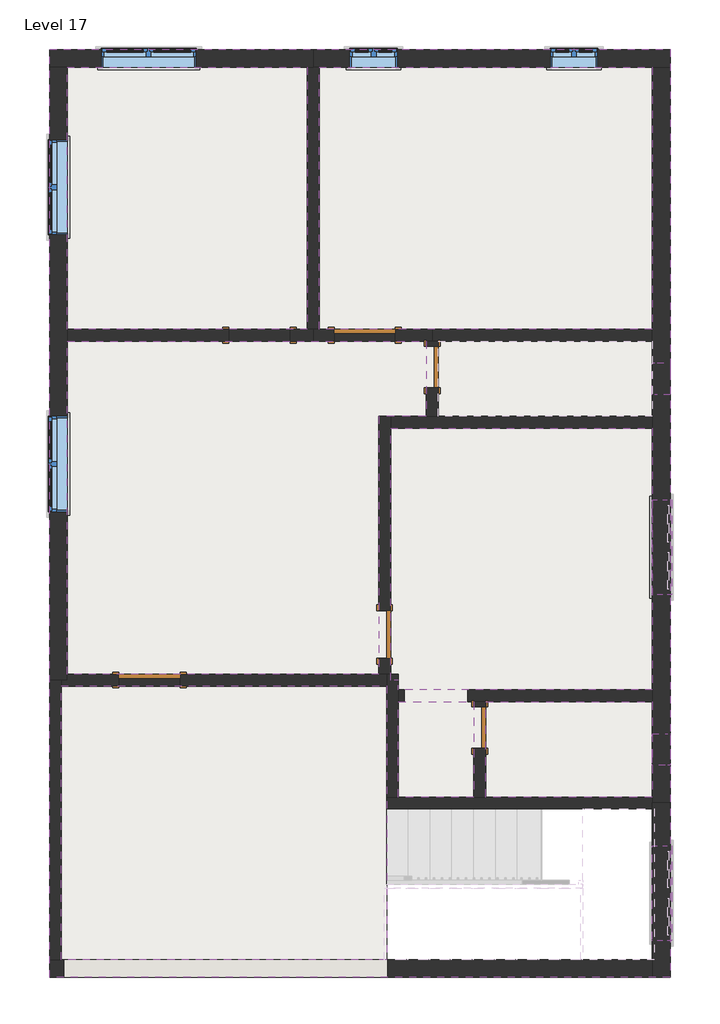
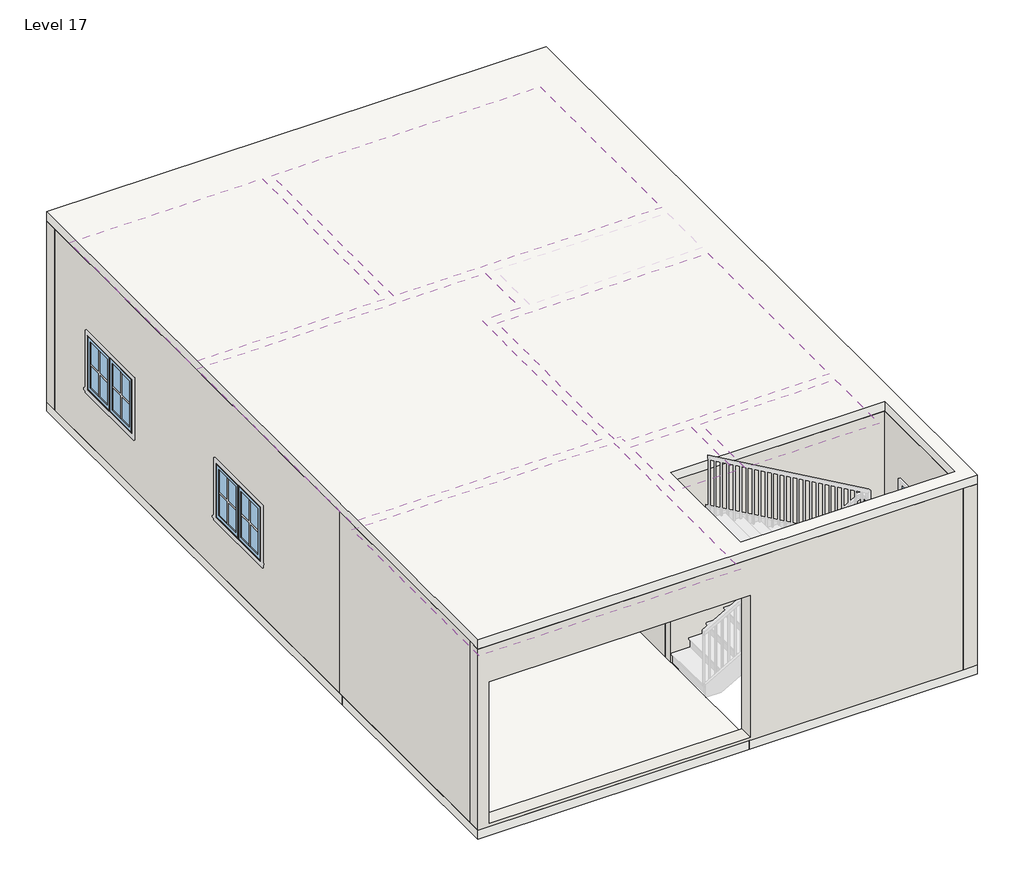
# One storey, part 1 of 2: 27 walls, 13 windows, 7 coverings, 6 doors, 3 slabs.
"""IFC4 building model written with IfcOpenShell, lengths in millimetres."""

from ifc_helpers import new_model, si_unit, frame, origin, place, context, project, spatial, polyline, outline, extrude, faceted_brep, transform, mapped, element, save
from components import door_2908be75, door_9ea4ff49, door_dc34e247, door_b804d09e, fixed_2_415b3208, window_casement_double_3_c417fced, window_casement_double_4_c19c33cb

model = new_model("IFC4")

# Units and contexts
model_context = context("Model", 3, world=origin())
ifc_project = project(units=[si_unit("LENGTHUNIT", "METRE", prefix="MILLI")], contexts=[model_context])

# Site, building, storey
site = spatial("IfcSite", under=ifc_project)
building = spatial("IfcBuilding", under=site)
storey = spatial("IfcBuildingStorey", under=building, Name="Level 17", Elevation=9601.2)

# Coverings
placement = place(None, origin())
element("IfcCovering", 1, ObjectType="2' x 4' ACT System", at=placement, inside=storey, context=model_context, shape_type="SweptSolid", body=[
    extrude(outline(polyline([(-5680.5154463, 2323.8455275), (-5680.5154463, 5678.2330275), (-2607.1154463, 5678.2330275), (-2607.1154463, 2323.8455275), (-5680.5154463, 2323.8455275)])), frame((0.0, 0.0, 12344.4), z_axis=(0.0, 0.0, 1.0), x_axis=(1.0, 0.0, 0.0)), (0.0, 0.0, 1.0), 57.15),
])
element("IfcCovering", 2, ObjectType="2' x 4' ACT System", at=placement, inside=storey, context=model_context, shape_type="SweptSolid", body=[
    extrude(outline(polyline([(-2454.7154463, 2323.8455275), (-2454.7154463, 5678.2330275), (1812.4845537, 5678.2330275), (1812.4845537, 2323.8455275), (-2454.7154463, 2323.8455275)])), frame((0.0, 0.0, 12344.4), z_axis=(0.0, 0.0, 1.0), x_axis=(1.0, 0.0, 0.0)), (0.0, 0.0, 1.0), 57.15),
])
element("IfcCovering", 3, ObjectType="2' x 4' ACT System", at=placement, inside=storey, context=model_context, shape_type="SweptSolid", body=[
    extrude(outline(polyline([(-5680.5154463, -2095.7544725), (-5680.5154463, 2171.4455275), (-1083.1154463, 2171.4455275), (-1083.1154463, 1206.2455275), (-1692.7154463, 1206.2455275), (-1692.7154463, -2095.7544725), (-5680.5154463, -2095.7544725)])), frame((0.0, 0.0, 12344.4), z_axis=(0.0, 0.0, 1.0), x_axis=(1.0, 0.0, 0.0)), (0.0, 0.0, 1.0), 57.15),
])
element("IfcCovering", 4, ObjectType="2' x 4' ACT System", at=placement, inside=storey, context=model_context, shape_type="SweptSolid", body=[
    extrude(outline(polyline([(1812.4845537, 1053.8455275), (1812.4845537, -2298.9544725), (-1438.7154463, -2298.9544725), (-1438.7154463, -2171.9544725), (-1540.3154463, -2171.9544725), (-1540.3154463, 1053.8455275), (1812.4845537, 1053.8455275)])), frame((0.0, 0.0, 12344.4), z_axis=(0.0, 0.0, 1.0), x_axis=(1.0, 0.0, 0.0)), (0.0, 0.0, 1.0), 57.15),
])
element("IfcCovering", 5, ObjectType="2' x 4' ACT System", at=placement, inside=storey, context=model_context, shape_type="SweptSolid", body=[
    extrude(outline(polyline([(1812.4845537, -2451.3544725), (1812.4845537, -3670.5544725), (-321.1154463, -3670.5544725), (-321.1154463, -2451.3544725), (1812.4845537, -2451.3544725)])), frame((0.0, 0.0, 12344.4), z_axis=(0.0, 0.0, 1.0), x_axis=(1.0, 0.0, 0.0)), (0.0, 0.0, 1.0), 57.15),
])
element("IfcCovering", 6, ObjectType="2' x 4' ACT System", at=placement, inside=storey, context=model_context, shape_type="SweptSolid", body=[
    extrude(outline(polyline([(-473.5154463, -2451.3544725), (-473.5154463, -3670.5544725), (-1438.7154463, -3670.5544725), (-1438.7154463, -2451.3544725), (-473.5154463, -2451.3544725)])), frame((0.0, 0.0, 12344.4), z_axis=(0.0, 0.0, 1.0), x_axis=(1.0, 0.0, 0.0)), (0.0, 0.0, 1.0), 57.15),
])
element("IfcCovering", 7, ObjectType="2' x 4' ACT System", at=placement, inside=storey, context=model_context, shape_type="SweptSolid", body=[
    extrude(outline(polyline([(-1591.1154463, -2248.1544725), (-1591.1154463, -5753.3544725), (-5756.7154463, -5753.3544725), (-5756.7154463, -2248.1544725), (-1591.1154463, -2248.1544725)])), frame((0.0, 0.0, 12344.4), z_axis=(0.0, 0.0, 1.0), x_axis=(1.0, 0.0, 0.0)), (0.0, 0.0, 1.0), 57.15),
])

# Doors
door_shape = door_2908be75(model_context)
element("IfcDoor", 8, ObjectType="Single-Flush : 1' 9\"", at=placement, inside=storey, context=model_context, shape_type="MappedRepresentation", body=[
    mapped(door_shape, transform((-397.3154463, -2781.5544725, 9601.2), x_axis=(0.0, 1.0, 0.0), y_axis=(-1.0, 0.0, 0.0), z_axis=(0.0, 0.0, 1.0))),
])
element("IfcDoor", 9, ObjectType="Single-Flush : 1' 9\"", at=placement, inside=storey, context=model_context, shape_type="MappedRepresentation", body=[
    mapped(door_shape, transform((-1006.9154463, 1841.2455275, 9601.2), x_axis=(0.0, 1.0, 0.0), y_axis=(-1.0, 0.0, 0.0), z_axis=(0.0, 0.0, 1.0))),
])
door_2_shape = door_9ea4ff49(model_context)
element("IfcDoor", 10, ObjectType="Single-Flush : 2'0\"", at=placement, inside=storey, context=model_context, shape_type="MappedRepresentation", body=[
    mapped(door_2_shape, transform((-1616.5154463, -1587.7544725, 9601.2), x_axis=(0.0, -1.0, 0.0), y_axis=(1.0, 0.0, 0.0), z_axis=(0.0, 0.0, 1.0))),
])
door_3_shape = door_dc34e247(model_context)
element("IfcDoor", 11, ObjectType="Single-Flush : 2'7\"", at=placement, inside=storey, context=model_context, shape_type="MappedRepresentation", body=[
    mapped(door_3_shape, transform((-4626.4154463, -2171.9544725, 9601.2), x_axis=(-1.0, 0.0, 0.0), y_axis=(0.0, -1.0, 0.0), z_axis=(0.0, 0.0, 1.0))),
])
element("IfcDoor", 12, ObjectType="Single-Flush : 2'7\"", at=placement, inside=storey, context=model_context, shape_type="MappedRepresentation", body=[
    mapped(door_3_shape, transform((-1870.5154463, 2247.6455275, 9601.2), x_axis=(-1.0, 0.0, 0.0), y_axis=(0.0, -1.0, 0.0), z_axis=(0.0, 0.0, 1.0))),
])
door_4_shape = door_b804d09e(model_context)
element("IfcDoor", 13, ObjectType="Single-Flush : 2'7\"", at=placement, inside=storey, context=model_context, shape_type="MappedRepresentation", body=[
    mapped(door_4_shape, transform((-3216.7154463, 2247.6455275, 9601.2), x_axis=(1.0, 0.0, 0.0), y_axis=(0.0, 1.0, 0.0), z_axis=(0.0, 0.0, 1.0))),
])

# Slabs
element("IfcSlab", 14, ObjectType="Generic - 6\"", at=placement, inside=storey, context=model_context, shape_type="SweptSolid", body=[
    extrude(outline(polyline([(-5909.1154463, -2248.1544725), (-5909.1154463, 5906.8330275), (2041.0845537, 5906.8330275), (2041.0845537, -5981.9544725), (-1591.1154463, -5981.9544725), (-1591.1154463, -5753.3544725), (1812.4845537, -5753.3544725), (1812.4845537, -3822.9544725), (-1591.1154463, -3822.9544725), (-1591.1154463, -2248.1544725), (-5756.7154463, -2248.1544725), (-5909.1154463, -2248.1544725)])), frame((0.0, 0.0, 9448.8), z_axis=(0.0, 0.0, 1.0), x_axis=(1.0, 0.0, 0.0)), (0.0, 0.0, 1.0), 152.4),
])
element("IfcSlab", 15, ObjectType="Generic - 6\"", at=placement, inside=storey, context=model_context, shape_type="SweptSolid", body=[
    extrude(outline(polyline([(-1591.1154463, -2248.1544725), (-1591.1154463, -5981.9544725), (-5909.1154463, -5981.9544725), (-5909.1154463, -2248.1544725), (-1591.1154463, -2248.1544725)])), frame((0.0, 0.0, 9448.8), z_axis=(0.0, 0.0, 1.0), x_axis=(1.0, 0.0, 0.0)), (0.0, 0.0, 1.0), 152.4),
])
element("IfcSlab", 16, ObjectType="Generic - 6\"", at=placement, inside=storey, context=model_context, shape_type="SweptSolid", body=[
    extrude(outline(polyline([(2041.0845537, 5906.8330275), (2041.0845537, -5981.9544725), (-5909.1154463, -5981.9544725), (-5909.1154463, 5906.8330275), (2041.0845537, 5906.8330275)]), holes=[polyline([(1812.4845537, -3822.9544725), (-1591.1154463, -3822.9544725), (-1591.1154463, -5753.3544725), (1812.4845537, -5753.3544725), (1812.4845537, -3822.9544725)])]), frame((0.0, 0.0, 12649.2), z_axis=(0.0, 0.0, 1.0), x_axis=(1.0, 0.0, 0.0)), (0.0, 0.0, 1.0), 152.4),
])

# Walls
element("IfcWall", 17, ObjectType="Generic - 6\"", at=placement, inside=storey, context=model_context, shape_type="Brep", body=[
    faceted_brep([(-5909.1154463, -2171.9544725, 9601.2), (-5909.1154463, -5753.3544725, 9601.2), (-5909.1154463, -5753.3544725, 12649.2), (-5909.1154463, -2171.9544725, 12649.2), (-5756.7154463, -2171.9544725, 9601.2), (-5756.7154463, -2171.9544725, 12649.2), (-5756.7154463, -2248.1544725, 12649.2), (-5756.7154463, -5753.3544725, 12649.2), (-5756.7154463, -5753.3544725, 9601.2), (-5756.7154463, -2248.1544725, 9601.2)], [[[0, 1, 2, 3]], [[4, 5, 6, 7, 8, 9]], [[1, 0, 4, 9, 8]], [[3, 2, 7, 6, 5]], [[0, 3, 5, 4]], [[2, 1, 8, 7]]]),
])
element("IfcWall", 18, ObjectType="Generic - 6\"", at=placement, inside=storey, context=model_context, shape_type="Brep", body=[
    faceted_brep([(1812.4845537, -3670.5544725, 9601.2), (-321.1154463, -3670.5544725, 9601.2), (-473.5154463, -3670.5544725, 9601.2), (-1438.7154463, -3670.5544725, 9601.2), (-1591.1154463, -3670.5544725, 9601.2), (-1591.1154463, -3670.5544725, 12649.2), (-1438.7154463, -3670.5544725, 12649.2), (-473.5154463, -3670.5544725, 12649.2), (-321.1154463, -3670.5544725, 12649.2), (1812.4845537, -3670.5544725, 12649.2), (1812.4845537, -3822.9544725, 9601.2), (1812.4845537, -3822.9544725, 12649.2), (-1591.1154463, -3822.9544725, 12649.2), (-1591.1154463, -3822.9544725, 9601.2), (1812.4845537, -3746.7544725, 9601.2), (1812.4845537, -3746.7544725, 12649.2)], [[[0, 1, 2, 3, 4, 5, 6, 7, 8, 9]], [[10, 11, 12, 13]], [[4, 3, 2, 1, 0, 14, 10, 13]], [[9, 8, 7, 6, 5, 12, 11, 15]], [[5, 4, 13, 12]], [[0, 9, 15, 11, 10, 14]]]),
])
element("IfcWall", 19, ObjectType="Generic - 6\"", at=placement, inside=storey, context=model_context, shape_type="Brep", body=[
    faceted_brep([(-1438.7154463, -3670.5544725, 9601.2), (-1438.7154463, -2451.3544725, 9601.2), (-1438.7154463, -2298.9544725, 9601.2), (-1438.7154463, -2095.7544725, 9601.2), (-1438.7154463, -2095.7544725, 12649.2), (-1438.7154463, -2298.9544725, 12649.2), (-1438.7154463, -2451.3544725, 12649.2), (-1438.7154463, -3670.5544725, 12649.2), (-1591.1154463, -3670.5544725, 9601.2), (-1591.1154463, -3670.5544725, 12649.2), (-1591.1154463, -2248.1544725, 12649.2), (-1591.1154463, -2171.9544725, 12649.2), (-1591.1154463, -2095.7544725, 12649.2), (-1591.1154463, -2095.7544725, 9601.2), (-1591.1154463, -2171.9544725, 9601.2), (-1591.1154463, -2248.1544725, 9601.2), (-1540.3154463, -2095.7544725, 9601.2), (-1540.3154463, -2095.7544725, 12649.2)], [[[0, 1, 2, 3, 4, 5, 6, 7]], [[8, 9, 10, 11, 12, 13, 14, 15]], [[3, 2, 1, 0, 8, 15, 14, 13, 16]], [[7, 6, 5, 4, 17, 12, 11, 10, 9]], [[0, 7, 9, 8]], [[4, 3, 16, 13, 12, 17]]]),
])
element("IfcWall", 20, ObjectType="Generic - 6\"", at=placement, inside=storey, context=model_context, shape_type="Brep", body=[
    faceted_brep([(-5020.1154463, -2095.7544725, 11734.8), (-5020.1154463, -2095.7544725, 9601.2), (-5680.5154463, -2095.7544725, 9601.2), (-5680.5154463, -2095.7544725, 12649.2), (-1692.7154463, -2095.7544725, 12649.2), (-1591.1154463, -2095.7544725, 12649.2), (-1591.1154463, -2095.7544725, 9601.2), (-1692.7154463, -2095.7544725, 9601.2), (-4232.7154463, -2095.7544725, 9601.2), (-4232.7154463, -2095.7544725, 11734.8), (-5756.7154463, -2248.1544725, 9601.2), (-5020.1154463, -2248.1544725, 9601.2), (-5020.1154463, -2248.1544725, 11734.8), (-4232.7154463, -2248.1544725, 11734.8), (-4232.7154463, -2248.1544725, 9601.2), (-1591.1154463, -2248.1544725, 9601.2), (-1591.1154463, -2248.1544725, 12649.2), (-5756.7154463, -2248.1544725, 12649.2), (-5756.7154463, -2171.9544725, 9601.2), (-5680.5154463, -2171.9544725, 9601.2), (-5680.5154463, -2171.9544725, 12649.2), (-5756.7154463, -2171.9544725, 12649.2)], [[[0, 1, 2, 3, 4, 5, 6, 7, 8, 9]], [[10, 11, 12, 13, 14, 15, 16, 17]], [[2, 1, 11, 10, 18, 19]], [[8, 7, 6, 15, 14]], [[5, 4, 3, 20, 21, 17, 16]], [[3, 2, 19, 20]], [[19, 18, 21, 20]], [[18, 10, 17, 21]], [[6, 5, 16, 15]], [[12, 11, 1, 0]], [[13, 12, 0, 9]], [[14, 13, 9, 8]]]),
])
element("IfcWall", 21, ObjectType="Generic - 6\"", at=placement, inside=storey, context=model_context, shape_type="Brep", body=[
    faceted_brep([(1812.4845537, -2451.3544725, 9601.2), (1812.4845537, -2451.3544725, 12649.2), (-321.1154463, -2451.3544725, 12649.2), (-473.5154463, -2451.3544725, 12649.2), (-1438.7154463, -2451.3544725, 12649.2), (-1438.7154463, -2451.3544725, 9601.2), (-1367.0206652, -2451.3544725, 9601.2), (-1367.0206652, -2451.3544725, 12039.6), (-547.4818767, -2451.3544725, 12039.6), (-547.4818767, -2451.3544725, 9601.2), (-473.5154463, -2451.3544725, 9601.2), (-321.1154463, -2451.3544725, 9601.2), (1812.4845537, -2298.9544725, 12649.2), (1812.4845537, -2298.9544725, 9601.2), (-547.4818767, -2298.9544725, 9601.2), (-547.4818767, -2298.9544725, 12039.6), (-1367.0206652, -2298.9544725, 12039.6), (-1367.0206652, -2298.9544725, 9601.2), (-1438.7154463, -2298.9544725, 9601.2), (-1438.7154463, -2298.9544725, 12649.2)], [[[0, 1, 2, 3, 4, 5, 6, 7, 8, 9, 10, 11]], [[12, 13, 14, 15, 16, 17, 18, 19]], [[5, 18, 17, 6]], [[13, 0, 11, 10, 9, 14]], [[4, 3, 2, 1, 12, 19]], [[1, 0, 13, 12]], [[5, 4, 19, 18]], [[7, 16, 15, 8]], [[16, 7, 6, 17]], [[8, 15, 14, 9]]]),
])
element("IfcWall", 22, ObjectType="Generic - 6\"", at=placement, inside=storey, context=model_context, shape_type="SweptSolid", body=[
    extrude(outline(polyline([(-2451.3544725, 9601.2), (-2514.8544725, 9601.2), (-2514.8544725, 11734.8), (-3048.2544725, 11734.8), (-3048.2544725, 9601.2), (-3670.5544725, 9601.2), (-3670.5544725, 12649.2), (-2451.3544725, 12649.2), (-2451.3544725, 9601.2)])), frame((-473.5154463, 0.0, 0.0), z_axis=(1.0, 0.0, 0.0), x_axis=(0.0, 1.0, 0.0)), (0.0, 0.0, 1.0), 152.4),
])
element("IfcWall", 23, ObjectType="Generic - 6\"", at=placement, inside=storey, context=model_context, shape_type="Brep", body=[
    faceted_brep([(-1540.3154463, -2095.7544725, 9601.2), (-1540.3154463, -1892.5544725, 9601.2), (-1540.3154463, -1892.5544725, 11734.8), (-1540.3154463, -1282.9544725, 11734.8), (-1540.3154463, -1282.9544725, 9601.2), (-1540.3154463, 1053.8455275, 9601.2), (-1540.3154463, 1206.2455275, 9601.2), (-1540.3154463, 1206.2455275, 12649.2), (-1540.3154463, 1053.8455275, 12649.2), (-1540.3154463, -2095.7544725, 12649.2), (-1692.7154463, -1892.5544725, 11734.8), (-1692.7154463, -1892.5544725, 9601.2), (-1692.7154463, -2095.7544725, 9601.2), (-1692.7154463, -2095.7544725, 12649.2), (-1692.7154463, 1206.2455275, 12649.2), (-1692.7154463, 1206.2455275, 9601.2), (-1692.7154463, -1282.9544725, 9601.2), (-1692.7154463, -1282.9544725, 11734.8), (-1591.1154463, -2095.7544725, 9601.2), (-1591.1154463, -2095.7544725, 12649.2)], [[[0, 1, 2, 3, 4, 5, 6, 7, 8, 9]], [[10, 11, 12, 13, 14, 15, 16, 17]], [[16, 15, 6, 5, 4]], [[12, 11, 1, 0, 18]], [[9, 8, 7, 14, 13, 19]], [[0, 9, 19, 13, 12, 18]], [[7, 6, 15, 14]], [[2, 1, 11, 10]], [[3, 2, 10, 17]], [[4, 3, 17, 16]]]),
])
element("IfcWall", 24, ObjectType="Generic - 6\"", at=placement, inside=storey, context=model_context, shape_type="Brep", body=[
    faceted_brep([(-1540.3154463, 1053.8455275, 9601.2), (1812.4845537, 1053.8455275, 9601.2), (1812.4845537, 1053.8455275, 12649.2), (-1540.3154463, 1053.8455275, 12649.2), (-1540.3154463, 1206.2455275, 9601.2), (-1540.3154463, 1206.2455275, 12649.2), (-1083.1154463, 1206.2455275, 12649.2), (-930.7154463, 1206.2455275, 12649.2), (1812.4845537, 1206.2455275, 12649.2), (1812.4845537, 1206.2455275, 9601.2), (-930.7154463, 1206.2455275, 9601.2), (-1083.1154463, 1206.2455275, 9601.2)], [[[0, 1, 2, 3]], [[4, 5, 6, 7, 8, 9, 10, 11]], [[1, 0, 4, 11, 10, 9]], [[3, 2, 8, 7, 6, 5]], [[0, 3, 5, 4]], [[2, 1, 9, 8]]]),
])
element("IfcWall", 25, ObjectType="Generic - 6\"", at=placement, inside=storey, context=model_context, shape_type="Brep", body=[
    faceted_brep([(-930.7154463, 2107.9455275, 11734.8), (-930.7154463, 2107.9455275, 9601.2), (-930.7154463, 2171.4455275, 9601.2), (-930.7154463, 2171.4455275, 12649.2), (-930.7154463, 1206.2455275, 12649.2), (-930.7154463, 1206.2455275, 9601.2), (-930.7154463, 1574.5455275, 9601.2), (-930.7154463, 1574.5455275, 11734.8), (-1083.1154463, 2171.4455275, 9601.2), (-1083.1154463, 2107.9455275, 9601.2), (-1083.1154463, 2107.9455275, 11734.8), (-1083.1154463, 1574.5455275, 11734.8), (-1083.1154463, 1574.5455275, 9601.2), (-1083.1154463, 1206.2455275, 9601.2), (-1083.1154463, 1206.2455275, 12649.2), (-1083.1154463, 2171.4455275, 12649.2), (-1006.9154463, 2171.4455275, 9601.2), (-1006.9154463, 2171.4455275, 12649.2)], [[[0, 1, 2, 3, 4, 5, 6, 7]], [[8, 9, 10, 11, 12, 13, 14, 15]], [[6, 5, 13, 12]], [[2, 1, 9, 8, 16]], [[4, 3, 17, 15, 14]], [[5, 4, 14, 13]], [[10, 9, 1, 0]], [[11, 10, 0, 7]], [[12, 11, 7, 6]], [[3, 2, 16, 8, 15, 17]]]),
])
element("IfcWall", 26, ObjectType="Generic - 6\"", at=placement, inside=storey, context=model_context, shape_type="Brep", body=[
    faceted_brep([(1812.4845537, 2323.8455275, 9601.2), (-1006.9154463, 2323.8455275, 9601.2), (-1006.9154463, 2323.8455275, 12649.2), (1812.4845537, 2323.8455275, 12649.2), (1812.4845537, 2171.4455275, 9601.2), (1812.4845537, 2171.4455275, 12649.2), (-930.7154463, 2171.4455275, 12649.2), (-1006.9154463, 2171.4455275, 12649.2), (-1006.9154463, 2171.4455275, 9601.2), (-930.7154463, 2171.4455275, 9601.2)], [[[0, 1, 2, 3]], [[4, 5, 6, 7, 8, 9]], [[1, 0, 4, 9, 8]], [[2, 1, 8, 7]], [[3, 2, 7, 6, 5]], [[0, 3, 5, 4]]]),
])
element("IfcWall", 27, ObjectType="Generic - 6\"", at=placement, inside=storey, context=model_context, shape_type="Brep", body=[
    faceted_brep([(-2607.1154463, 5678.2330275, 9601.2), (-2607.1154463, 2323.8455275, 9601.2), (-2607.1154463, 2323.8455275, 12649.2), (-2607.1154463, 5678.2330275, 12649.2), (-2454.7154463, 5678.2330275, 9601.2), (-2454.7154463, 5678.2330275, 12649.2), (-2454.7154463, 2323.8455275, 12649.2), (-2454.7154463, 2323.8455275, 9601.2), (-2530.9154463, 5678.2330275, 9601.2), (-2530.9154463, 2323.8455275, 9601.2), (-2530.9154463, 2323.8455275, 12649.2), (-2530.9154463, 5678.2330275, 12649.2)], [[[0, 1, 2, 3]], [[4, 5, 6, 7]], [[1, 0, 8, 4, 7, 9]], [[3, 2, 10, 6, 5, 11]], [[0, 3, 11, 5, 4, 8]], [[2, 1, 9, 7, 6, 10]]]),
])
element("IfcWall", 28, ObjectType="Generic - 6\"", at=placement, inside=storey, context=model_context, shape_type="Brep", body=[
    faceted_brep([(-2530.9154463, 2323.8455275, 9601.2), (-2607.1154463, 2323.8455275, 9601.2), (-2823.0154463, 2323.8455275, 9601.2), (-2823.0154463, 2323.8455275, 11734.8), (-3610.4154463, 2323.8455275, 11734.8), (-3610.4154463, 2323.8455275, 9601.2), (-5680.5154463, 2323.8455275, 9601.2), (-5680.5154463, 2323.8455275, 12649.2), (-2607.1154463, 2323.8455275, 12649.2), (-2530.9154463, 2323.8455275, 12649.2), (-2823.0154463, 2171.4455275, 11734.8), (-2823.0154463, 2171.4455275, 9601.2), (-2530.9154463, 2171.4455275, 9601.2), (-2530.9154463, 2171.4455275, 12649.2), (-5680.5154463, 2171.4455275, 12649.2), (-5680.5154463, 2171.4455275, 9601.2), (-3610.4154463, 2171.4455275, 9601.2), (-3610.4154463, 2171.4455275, 11734.8)], [[[0, 1, 2, 3, 4, 5, 6, 7, 8, 9]], [[10, 11, 12, 13, 14, 15, 16, 17]], [[16, 15, 6, 5]], [[12, 11, 2, 1, 0]], [[9, 8, 7, 14, 13]], [[0, 9, 13, 12]], [[7, 6, 15, 14]], [[5, 4, 17, 16]], [[4, 3, 10, 17]], [[3, 2, 11, 10]]]),
])
element("IfcWall", 29, ObjectType="Generic - 6\"", at=placement, inside=storey, context=model_context, shape_type="Brep", body=[
    faceted_brep([(-2264.2154463, 2323.8455275, 11734.8), (-2264.2154463, 2323.8455275, 9601.2), (-2454.7154463, 2323.8455275, 9601.2), (-2530.9154463, 2323.8455275, 9601.2), (-2530.9154463, 2323.8455275, 12649.2), (-2454.7154463, 2323.8455275, 12649.2), (-1006.9154463, 2323.8455275, 12649.2), (-1006.9154463, 2323.8455275, 9601.2), (-1476.8154463, 2323.8455275, 9601.2), (-1476.8154463, 2323.8455275, 11734.8), (-2530.9154463, 2171.4455275, 9601.2), (-2264.2154463, 2171.4455275, 9601.2), (-2264.2154463, 2171.4455275, 11734.8), (-1476.8154463, 2171.4455275, 11734.8), (-1476.8154463, 2171.4455275, 9601.2), (-1083.1154463, 2171.4455275, 9601.2), (-1006.9154463, 2171.4455275, 9601.2), (-1006.9154463, 2171.4455275, 12649.2), (-1083.1154463, 2171.4455275, 12649.2), (-2530.9154463, 2171.4455275, 12649.2)], [[[0, 1, 2, 3, 4, 5, 6, 7, 8, 9]], [[10, 11, 12, 13, 14, 15, 16, 17, 18, 19]], [[8, 7, 16, 15, 14]], [[3, 2, 1, 11, 10]], [[4, 3, 10, 19]], [[6, 5, 4, 19, 18, 17]], [[7, 6, 17, 16]], [[14, 13, 9, 8]], [[13, 12, 0, 9]], [[12, 11, 1, 0]]]),
])
element("IfcWall", 30, ObjectType="Generic - 6\"", at=placement, inside=storey, context=model_context, shape_type="SweptSolid", body=[
    extrude(outline(polyline([(-5680.5154463, -2095.7544725), (-1692.7154463, -2095.7544725), (-1692.7154463, -2171.9544725), (-1591.1154463, -2171.9544725), (-1591.1154463, -2248.1544725), (-5756.7154463, -2248.1544725), (-5756.7154463, -2171.9544725), (-5680.5154463, -2171.9544725), (-5680.5154463, -2095.7544725)])), frame((0.0, 0.0, 9601.2), z_axis=(0.0, 0.0, 1.0), x_axis=(1.0, 0.0, 0.0)), (0.0, 0.0, 1.0), 3048.0),
])
element("IfcWall", 31, ObjectType="Generic - 6\"", at=placement, inside=storey, context=model_context, shape_type="Brep", body=[
    faceted_brep([(-2607.1154463, 5678.2330275, 9601.2), (-2607.1154463, 2323.8455275, 9601.2), (-2607.1154463, 2323.8455275, 12649.2), (-2607.1154463, 5678.2330275, 12649.2), (-2454.7154463, 5678.2330275, 9601.2), (-2454.7154463, 5678.2330275, 12649.2), (-2454.7154463, 2323.8455275, 12649.2), (-2454.7154463, 2323.8455275, 9601.2), (-2530.9154463, 5678.2330275, 9601.2), (-2530.9154463, 2323.8455275, 9601.2), (-2530.9154463, 2323.8455275, 12649.2), (-2530.9154463, 5678.2330275, 12649.2)], [[[0, 1, 2, 3]], [[4, 5, 6, 7]], [[1, 0, 8, 4, 7, 9]], [[3, 2, 10, 6, 5, 11]], [[0, 3, 11, 5, 4, 8]], [[2, 1, 9, 7, 6, 10]]]),
])
element("IfcWall", 32, ObjectType="Generic - 6\"", at=placement, inside=storey, context=model_context, shape_type="Brep", body=[
    faceted_brep([(-2530.9154463, 2323.8455275, 9601.2), (-2607.1154463, 2323.8455275, 9601.2), (-5680.5154463, 2323.8455275, 9601.2), (-5680.5154463, 2323.8455275, 12649.2), (-2607.1154463, 2323.8455275, 12649.2), (-2530.9154463, 2323.8455275, 12649.2), (-2530.9154463, 2171.4455275, 9601.2), (-2530.9154463, 2171.4455275, 12649.2), (-5680.5154463, 2171.4455275, 12649.2), (-5680.5154463, 2171.4455275, 9601.2)], [[[0, 1, 2, 3, 4, 5]], [[6, 7, 8, 9]], [[2, 1, 0, 6, 9]], [[5, 4, 3, 8, 7]], [[0, 5, 7, 6]], [[3, 2, 9, 8]]]),
])
element("IfcWall", 33, ObjectType="Generic - 6\"", at=placement, inside=storey, context=model_context, shape_type="Brep", body=[
    faceted_brep([(-1006.9154463, 2323.8455275, 9601.2), (-2454.7154463, 2323.8455275, 9601.2), (-2530.9154463, 2323.8455275, 9601.2), (-2530.9154463, 2323.8455275, 12649.2), (-2454.7154463, 2323.8455275, 12649.2), (-1006.9154463, 2323.8455275, 12649.2), (-1006.9154463, 2171.4455275, 9601.2), (-1006.9154463, 2171.4455275, 12649.2), (-1083.1154463, 2171.4455275, 12649.2), (-2530.9154463, 2171.4455275, 12649.2), (-2530.9154463, 2171.4455275, 9601.2), (-1083.1154463, 2171.4455275, 9601.2)], [[[0, 1, 2, 3, 4, 5]], [[6, 7, 8, 9, 10, 11]], [[2, 1, 0, 6, 11, 10]], [[3, 2, 10, 9]], [[5, 4, 3, 9, 8, 7]], [[0, 5, 7, 6]]]),
])
element("IfcWall", 34, ObjectType="Generic - 9\"", at=placement, inside=storey, context=model_context, shape_type="Brep", body=[
    faceted_brep([(-5909.1154463, 5678.2330275, 9601.2), (-5680.5154463, 5678.2330275, 9601.2), (-2607.1154463, 5678.2330275, 9601.2), (-2530.9154463, 5678.2330275, 9601.2), (-2530.9154463, 5678.2330275, 12649.2), (-2607.1154463, 5678.2330275, 12649.2), (-5680.5154463, 5678.2330275, 12649.2), (-5909.1154463, 5678.2330275, 12649.2), (-4029.5154463, 5678.2330275, 11430.0), (-4029.5154463, 5678.2330275, 10515.6), (-5248.7154463, 5678.2330275, 10515.6), (-5248.7154463, 5678.2330275, 11430.0), (-5909.1154463, 5906.8330275, 9601.2), (-5909.1154463, 5906.8330275, 12649.2), (-2530.9154463, 5906.8330275, 12649.2), (-2530.9154463, 5906.8330275, 9601.2), (-4029.5154463, 5906.8330275, 11430.0), (-5248.7154463, 5906.8330275, 11430.0), (-5248.7154463, 5906.8330275, 10515.6), (-4029.5154463, 5906.8330275, 10515.6)], [[[0, 1, 2, 3, 4, 5, 6, 7], [8, 9, 10, 11]], [[12, 13, 14, 15], [16, 17, 18, 19]], [[3, 2, 1, 0, 12, 15]], [[4, 3, 15, 14]], [[7, 6, 5, 4, 14, 13]], [[0, 7, 13, 12]], [[9, 8, 16, 19]], [[10, 9, 19, 18]], [[11, 10, 18, 17]], [[8, 11, 17, 16]]]),
])
element("IfcWall", 35, ObjectType="Generic - 9\"", at=placement, inside=storey, context=model_context, shape_type="Brep", body=[
    faceted_brep([(1812.4845537, 5678.2330275, 9601.2), (1812.4845537, 2323.8455275, 9601.2), (1812.4845537, 2171.4455275, 9601.2), (1812.4845537, 1206.2455275, 9601.2), (1812.4845537, 1053.8455275, 9601.2), (1812.4845537, -2298.9544725, 9601.2), (1812.4845537, -2451.3544725, 9601.2), (1812.4845537, -3670.5544725, 9601.2), (1812.4845537, -3746.7544725, 9601.2), (1812.4845537, -3746.7544725, 12649.2), (1812.4845537, -3670.5544725, 12649.2), (1812.4845537, -2451.3544725, 12649.2), (1812.4845537, -2298.9544725, 12649.2), (1812.4845537, 1053.8455275, 12649.2), (1812.4845537, 1206.2455275, 12649.2), (1812.4845537, 2171.4455275, 12649.2), (1812.4845537, 2323.8455275, 12649.2), (1812.4845537, 5678.2330275, 12649.2), (1812.4845537, -1079.7544725, 11734.8), (1812.4845537, -1079.7544725, 10820.4), (1812.4845537, 139.4455275, 10820.4), (1812.4845537, 139.4455275, 11734.8), (1812.4845537, -3264.1544725, 12039.6), (1812.4845537, -3264.1544725, 11430.0), (1812.4845537, -2857.7544725, 11430.0), (1812.4845537, -2857.7544725, 12039.6), (1812.4845537, 1892.0455275, 12039.6), (1812.4845537, 1485.6455275, 12039.6), (1812.4845537, 1485.6455275, 11430.0), (1812.4845537, 1892.0455275, 11430.0), (2041.0845537, 5678.2330275, 9601.2), (2041.0845537, 5678.2330275, 12649.2), (2041.0845537, -3746.7544725, 12649.2), (2041.0845537, -3746.7544725, 9601.2), (2041.0845537, -1079.7544725, 11734.8), (2041.0845537, 139.4455275, 11734.8), (2041.0845537, 139.4455275, 10820.4), (2041.0845537, -1079.7544725, 10820.4), (2041.0845537, -3264.1544725, 12039.6), (2041.0845537, -2857.7544725, 12039.6), (2041.0845537, -2857.7544725, 11430.0), (2041.0845537, -3264.1544725, 11430.0), (2041.0845537, 1892.0455275, 12039.6), (2041.0845537, 1892.0455275, 11430.0), (2041.0845537, 1485.6455275, 11430.0), (2041.0845537, 1485.6455275, 12039.6)], [[[0, 1, 2, 3, 4, 5, 6, 7, 8, 9, 10, 11, 12, 13, 14, 15, 16, 17], [18, 19, 20, 21], [22, 23, 24, 25], [26, 27, 28, 29]], [[30, 31, 32, 33], [34, 35, 36, 37], [38, 39, 40, 41], [42, 43, 44, 45]], [[8, 7, 6, 5, 4, 3, 2, 1, 0, 30, 33]], [[9, 8, 33, 32]], [[17, 16, 15, 14, 13, 12, 11, 10, 9, 32, 31]], [[0, 17, 31, 30]], [[19, 18, 34, 37]], [[20, 19, 37, 36]], [[21, 20, 36, 35]], [[18, 21, 35, 34]], [[23, 22, 38, 41]], [[24, 23, 41, 40]], [[25, 24, 40, 39]], [[22, 25, 39, 38]], [[43, 42, 26, 29]], [[44, 43, 29, 28]], [[45, 44, 28, 27]], [[42, 45, 27, 26]]]),
])
element("IfcWall", 36, ObjectType="Generic - 9\"", at=placement, inside=storey, context=model_context, shape_type="Brep", body=[
    faceted_brep([(1812.4845537, -5753.3544725, 9601.2), (-5756.7154463, -5753.3544725, 9601.2), (-5909.1154463, -5753.3544725, 9601.2), (-5909.1154463, -5753.3544725, 12649.2), (-5756.7154463, -5753.3544725, 12649.2), (1812.4845537, -5753.3544725, 12649.2), (-1576.8982041, -5753.3544725, 12039.6), (-5729.1673724, -5753.3544725, 12039.6), (-5729.1673724, -5753.3544725, 9652.0), (-1576.8982041, -5753.3544725, 9652.0), (-5909.1154463, -5981.9544725, 9601.2), (1812.4845537, -5981.9544725, 9601.2), (1812.4845537, -5981.9544725, 12649.2), (-5909.1154463, -5981.9544725, 12649.2), (-5729.1673724, -5981.9544725, 12039.6), (-1576.8982041, -5981.9544725, 12039.6), (-1576.8982041, -5981.9544725, 9652.0), (-5729.1673724, -5981.9544725, 9652.0)], [[[0, 1, 2, 3, 4, 5], [6, 7, 8, 9]], [[10, 11, 12, 13], [14, 15, 16, 17]], [[2, 1, 0, 11, 10]], [[5, 4, 3, 13, 12]], [[0, 5, 12, 11]], [[6, 15, 14, 7]], [[8, 17, 16, 9]], [[15, 6, 9, 16]], [[7, 14, 17, 8]], [[3, 2, 10, 13]]]),
])
element("IfcWall", 37, ObjectType="Generic - 9\"", at=placement, inside=storey, context=model_context, shape_type="Brep", body=[
    faceted_brep([(-5909.1154463, 5678.2330275, 9601.2), (-5909.1154463, -2171.9544725, 9601.2), (-5909.1154463, -2171.9544725, 12649.2), (-5909.1154463, 5678.2330275, 12649.2), (-5909.1154463, 4751.1330275, 11430.0), (-5909.1154463, 3531.9330275, 11430.0), (-5909.1154463, 3531.9330275, 10515.6), (-5909.1154463, 4751.1330275, 10515.6), (-5909.1154463, 1206.2455275, 11430.0), (-5909.1154463, -12.9544725, 11430.0), (-5909.1154463, -12.9544725, 10515.6), (-5909.1154463, 1206.2455275, 10515.6), (-5680.5154463, 5678.2330275, 9601.2), (-5680.5154463, 5678.2330275, 12649.2), (-5680.5154463, 2323.8455275, 12649.2), (-5680.5154463, 2171.4455275, 12649.2), (-5680.5154463, -2095.7544725, 12649.2), (-5680.5154463, -2171.9544725, 12649.2), (-5680.5154463, -2171.9544725, 9601.2), (-5680.5154463, -2095.7544725, 9601.2), (-5680.5154463, 2171.4455275, 9601.2), (-5680.5154463, 2323.8455275, 9601.2), (-5680.5154463, 4751.1330275, 11430.0), (-5680.5154463, 4751.1330275, 10515.6), (-5680.5154463, 3531.9330275, 10515.6), (-5680.5154463, 3531.9330275, 11430.0), (-5680.5154463, 1206.2455275, 11430.0), (-5680.5154463, 1206.2455275, 10515.6), (-5680.5154463, -12.9544725, 10515.6), (-5680.5154463, -12.9544725, 11430.0), (-5756.7154463, -2171.9544725, 9601.2), (-5756.7154463, -2171.9544725, 12649.2)], [[[0, 1, 2, 3], [4, 5, 6, 7], [8, 9, 10, 11]], [[12, 13, 14, 15, 16, 17, 18, 19, 20, 21], [22, 23, 24, 25], [26, 27, 28, 29]], [[1, 0, 12, 21, 20, 19, 18, 30]], [[2, 1, 30, 18, 17, 31]], [[3, 2, 31, 17, 16, 15, 14, 13]], [[0, 3, 13, 12]], [[23, 22, 4, 7]], [[24, 23, 7, 6]], [[25, 24, 6, 5]], [[22, 25, 5, 4]], [[27, 26, 8, 11]], [[28, 27, 11, 10]], [[29, 28, 10, 9]], [[26, 29, 9, 8]]]),
])
element("IfcWall", 38, ObjectType="Generic - 9\"", at=placement, inside=storey, context=model_context, shape_type="Brep", body=[
    faceted_brep([(-2530.9154463, 5678.2330275, 9601.2), (-2454.7154463, 5678.2330275, 9601.2), (1812.4845537, 5678.2330275, 9601.2), (2041.0845537, 5678.2330275, 9601.2), (2041.0845537, 5678.2330275, 12649.2), (1812.4845537, 5678.2330275, 12649.2), (-2454.7154463, 5678.2330275, 12649.2), (-2530.9154463, 5678.2330275, 12649.2), (-1451.4154463, 5678.2330275, 11430.0), (-1451.4154463, 5678.2330275, 10515.6), (-2061.0154463, 5678.2330275, 10515.6), (-2061.0154463, 5678.2330275, 11430.0), (1113.9845537, 5678.2330275, 11430.0), (1113.9845537, 5678.2330275, 10515.6), (504.3845537, 5678.2330275, 10515.6), (504.3845537, 5678.2330275, 11430.0), (-2530.9154463, 5906.8330275, 9601.2), (-2530.9154463, 5906.8330275, 12649.2), (2041.0845537, 5906.8330275, 12649.2), (2041.0845537, 5906.8330275, 9601.2), (-1451.4154463, 5906.8330275, 11430.0), (-2061.0154463, 5906.8330275, 11430.0), (-2061.0154463, 5906.8330275, 10515.6), (-1451.4154463, 5906.8330275, 10515.6), (1113.9845537, 5906.8330275, 11430.0), (504.3845537, 5906.8330275, 11430.0), (504.3845537, 5906.8330275, 10515.6), (1113.9845537, 5906.8330275, 10515.6)], [[[0, 1, 2, 3, 4, 5, 6, 7], [8, 9, 10, 11], [12, 13, 14, 15]], [[16, 17, 18, 19], [20, 21, 22, 23], [24, 25, 26, 27]], [[3, 2, 1, 0, 16, 19]], [[7, 6, 5, 4, 18, 17]], [[0, 7, 17, 16]], [[4, 3, 19, 18]], [[8, 11, 21, 20]], [[11, 10, 22, 21]], [[10, 9, 23, 22]], [[9, 8, 20, 23]], [[12, 15, 25, 24]], [[15, 14, 26, 25]], [[14, 13, 27, 26]], [[13, 12, 24, 27]]]),
])
element("IfcWall", 39, ObjectType="Generic - 9\"", at=placement, inside=storey, context=model_context, shape_type="Brep", body=[
    faceted_brep([(1812.4845537, -3746.7544725, 9601.2), (1812.4845537, -3822.9544725, 9601.2), (1812.4845537, -5753.3544725, 9601.2), (1812.4845537, -5981.9544725, 9601.2), (1812.4845537, -5981.9544725, 12649.2), (1812.4845537, -5753.3544725, 12649.2), (1812.4845537, -3822.9544725, 12649.2), (1812.4845537, -3746.7544725, 12649.2), (1812.4845537, -5512.0544725, 11734.8), (1812.4845537, -5512.0544725, 10820.4), (1812.4845537, -4292.8544725, 10820.4), (1812.4845537, -4292.8544725, 11734.8), (2041.0845537, -3746.7544725, 9601.2), (2041.0845537, -3746.7544725, 12649.2), (2041.0845537, -5981.9544725, 12649.2), (2041.0845537, -5981.9544725, 9601.2), (2041.0845537, -5512.0544725, 11734.8), (2041.0845537, -4292.8544725, 11734.8), (2041.0845537, -4292.8544725, 10820.4), (2041.0845537, -5512.0544725, 10820.4)], [[[0, 1, 2, 3, 4, 5, 6, 7], [8, 9, 10, 11]], [[12, 13, 14, 15], [16, 17, 18, 19]], [[3, 2, 1, 0, 12, 15]], [[7, 6, 5, 4, 14, 13]], [[0, 7, 13, 12]], [[4, 3, 15, 14]], [[8, 11, 17, 16]], [[11, 10, 18, 17]], [[10, 9, 19, 18]], [[9, 8, 16, 19]]]),
])
element("IfcWall", 40, ObjectType="Generic - 9\"", at=placement, inside=storey, context=model_context, shape_type="SweptSolid", body=[
    extrude(outline(polyline([(9601.2, -5680.5154463), (9601.2, -2607.1154463), (12649.2, -2607.1154463), (12649.2, -5680.5154463), (9601.2, -5680.5154463)]), holes=[polyline([(11430.0, -4029.5154463), (10515.6, -4029.5154463), (10515.6, -5248.7154463), (11430.0, -5248.7154463), (11430.0, -4029.5154463)])]), frame((0.0, 5678.2330275, 0.0), z_axis=(0.0, 1.0, 0.0), x_axis=(0.0, 0.0, 1.0)), (0.0, 0.0, 1.0), 228.6),
])
element("IfcWall", 41, ObjectType="Generic - 9\"", at=placement, inside=storey, context=model_context, shape_type="Brep", body=[
    faceted_brep([(1812.4845537, -5753.3544725, 9601.2), (-5756.7154463, -5753.3544725, 9601.2), (-5909.1154463, -5753.3544725, 9601.2), (-5909.1154463, -5753.3544725, 12649.2), (-5756.7154463, -5753.3544725, 12649.2), (1812.4845537, -5753.3544725, 12649.2), (-1576.8982041, -5753.3544725, 12039.6), (-5729.1673724, -5753.3544725, 12039.6), (-5729.1673724, -5753.3544725, 9652.0), (-1576.8982041, -5753.3544725, 9652.0), (-5909.1154463, -5981.9544725, 9601.2), (1812.4845537, -5981.9544725, 9601.2), (1812.4845537, -5981.9544725, 12649.2), (-5909.1154463, -5981.9544725, 12649.2), (-5729.1673724, -5981.9544725, 12039.6), (-1576.8982041, -5981.9544725, 12039.6), (-1576.8982041, -5981.9544725, 9652.0), (-5729.1673724, -5981.9544725, 9652.0)], [[[0, 1, 2, 3, 4, 5], [6, 7, 8, 9]], [[10, 11, 12, 13], [14, 15, 16, 17]], [[2, 1, 0, 11, 10]], [[5, 4, 3, 13, 12]], [[6, 15, 14, 7]], [[8, 17, 16, 9]], [[15, 6, 9, 16]], [[7, 14, 17, 8]], [[3, 2, 10, 13]], [[0, 5, 12, 11]]]),
])
element("IfcWall", 42, ObjectType="Generic - 9\"", at=placement, inside=storey, context=model_context, shape_type="SweptSolid", body=[
    extrude(outline(polyline([(9601.2, -2454.7154463), (9601.2, 1812.4845537), (12649.2, 1812.4845537), (12649.2, -2454.7154463), (9601.2, -2454.7154463)]), holes=[polyline([(11430.0, -1451.4154463), (10515.6, -1451.4154463), (10515.6, -2061.0154463), (11430.0, -2061.0154463), (11430.0, -1451.4154463)]), polyline([(11430.0, 1113.9845537), (10515.6, 1113.9845537), (10515.6, 504.3845537), (11430.0, 504.3845537), (11430.0, 1113.9845537)])]), frame((0.0, 5678.2330275, 0.0), z_axis=(0.0, 1.0, 0.0), x_axis=(0.0, 0.0, 1.0)), (0.0, 0.0, 1.0), 228.6),
])
element("IfcWall", 43, ObjectType="Generic - 9\"", at=placement, inside=storey, context=model_context, shape_type="SweptSolid", body=[
    extrude(outline(polyline([(-3822.9544725, 9601.2), (-5753.3544725, 9601.2), (-5753.3544725, 12649.2), (-3822.9544725, 12649.2), (-3822.9544725, 9601.2)]), holes=[polyline([(-5512.0544725, 11734.8), (-5512.0544725, 10820.4), (-4292.8544725, 10820.4), (-4292.8544725, 11734.8), (-5512.0544725, 11734.8)])]), frame((1812.4845537, 0.0, 0.0), z_axis=(1.0, 0.0, 0.0), x_axis=(0.0, 1.0, 0.0)), (0.0, 0.0, 1.0), 228.6),
])

# Windows
fixed_2_shape = fixed_2_415b3208(model_context)
element("IfcWindow", 44, ObjectType="Fixed : 2'", at=placement, inside=storey, context=model_context, shape_type="MappedRepresentation", body=[
    mapped(fixed_2_shape, transform((1926.7845537, -3099.0544725, 11125.2), x_axis=(0.0, -1.0, 0.0), y_axis=(1.0, 0.0, 0.0), z_axis=(0.0, 0.0, 1.0))),
])
element("IfcWindow", 45, ObjectType="Fixed : 2'", at=placement, inside=storey, context=model_context, shape_type="MappedRepresentation", body=[
    mapped(fixed_2_shape, transform((1926.7845537, 1726.9455275, 11125.2), x_axis=(0.0, 1.0, 0.0), y_axis=(-1.0, 0.0, 0.0), z_axis=(0.0, 0.0, 1.0))),
])
window_casement_double_3_shape = window_casement_double_3_c417fced(model_context)
element("IfcWindow", 46, ObjectType="Window-Casement-Double : 3'", at=placement, inside=storey, context=model_context, shape_type="MappedRepresentation", body=[
    mapped(window_casement_double_3_shape, transform((-1756.2154463, 5792.5330275, 9601.2), x_axis=(1.0, 0.0, 0.0), y_axis=(0.0, 1.0, 0.0), z_axis=(0.0, 0.0, 1.0))),
])
element("IfcWindow", 47, ObjectType="Window-Casement-Double : 3'", at=placement, inside=storey, context=model_context, shape_type="MappedRepresentation", body=[
    mapped(window_casement_double_3_shape, transform((809.1845537, 5792.5330275, 9601.2), x_axis=(1.0, 0.0, 0.0), y_axis=(0.0, 1.0, 0.0), z_axis=(0.0, 0.0, 1.0))),
])
element("IfcWindow", 48, ObjectType="Window-Casement-Double : 3'", at=placement, inside=storey, context=model_context, shape_type="MappedRepresentation", body=[
    mapped(window_casement_double_3_shape, transform((-1756.2154463, 5792.5330275, 9601.2), x_axis=(1.0, 0.0, 0.0), y_axis=(0.0, 1.0, 0.0), z_axis=(0.0, 0.0, 1.0))),
])
element("IfcWindow", 49, ObjectType="Window-Casement-Double : 3'", at=placement, inside=storey, context=model_context, shape_type="MappedRepresentation", body=[
    mapped(window_casement_double_3_shape, transform((809.1845537, 5792.5330275, 9601.2), x_axis=(1.0, 0.0, 0.0), y_axis=(0.0, 1.0, 0.0), z_axis=(0.0, 0.0, 1.0))),
])
window_casement_double_4_shape = window_casement_double_4_c19c33cb(model_context)
element("IfcWindow", 50, ObjectType="Window-Casement-Double : 4'", at=placement, inside=storey, context=model_context, shape_type="MappedRepresentation", body=[
    mapped(window_casement_double_4_shape, transform((-4639.1154463, 5792.5330275, 9601.2), x_axis=(1.0, 0.0, 0.0), y_axis=(0.0, 1.0, 0.0), z_axis=(0.0, 0.0, 1.0))),
])
element("IfcWindow", 51, ObjectType="Window-Casement-Double : 4'", at=placement, inside=storey, context=model_context, shape_type="MappedRepresentation", body=[
    mapped(window_casement_double_4_shape, transform((-5794.8154463, 4141.5330275, 9601.2), x_axis=(0.0, 1.0, 0.0), y_axis=(-1.0, 0.0, 0.0), z_axis=(0.0, 0.0, 1.0))),
])
element("IfcWindow", 52, ObjectType="Window-Casement-Double : 4'", at=placement, inside=storey, context=model_context, shape_type="MappedRepresentation", body=[
    mapped(window_casement_double_4_shape, transform((-5794.8154463, 596.6455275, 9601.2), x_axis=(0.0, 1.0, 0.0), y_axis=(-1.0, 0.0, 0.0), z_axis=(0.0, 0.0, 1.0))),
])
element("IfcWindow", 53, ObjectType="Window-Casement-Double : 4'", at=placement, inside=storey, context=model_context, shape_type="MappedRepresentation", body=[
    mapped(window_casement_double_4_shape, transform((1926.7845537, -470.1544725, 9906.0), x_axis=(0.0, -1.0, 0.0), y_axis=(1.0, 0.0, 0.0), z_axis=(0.0, 0.0, 1.0))),
])
element("IfcWindow", 54, ObjectType="Window-Casement-Double : 4'", at=placement, inside=storey, context=model_context, shape_type="MappedRepresentation", body=[
    mapped(window_casement_double_4_shape, transform((1926.7845537, -4902.4544725, 9906.0), x_axis=(0.0, -1.0, 0.0), y_axis=(1.0, 0.0, 0.0), z_axis=(0.0, 0.0, 1.0))),
])
element("IfcWindow", 55, ObjectType="Window-Casement-Double : 4'", at=placement, inside=storey, context=model_context, shape_type="MappedRepresentation", body=[
    mapped(window_casement_double_4_shape, transform((-4639.1154463, 5792.5330275, 9601.2), x_axis=(1.0, 0.0, 0.0), y_axis=(0.0, 1.0, 0.0), z_axis=(0.0, 0.0, 1.0))),
])
element("IfcWindow", 56, ObjectType="Window-Casement-Double : 4'", at=placement, inside=storey, context=model_context, shape_type="MappedRepresentation", body=[
    mapped(window_casement_double_4_shape, transform((1926.7845537, -4902.4544725, 9906.0), x_axis=(0.0, -1.0, 0.0), y_axis=(1.0, 0.0, 0.0), z_axis=(0.0, 0.0, 1.0))),
])

save(model, "model.ifc")

# Revit data of these elements
# Type "2' x 4' ACT System"
#   Assembly Code = "C3030210"
#   built-in parameter 1002203 = 1 (stored number, unit not read)
#   built-in parameter 1002202 = 1 (stored number, unit not read)
#   Layers, outside or top first: 0' - 1 5/8" "Default" (function 1); 0' - 0 5/8" "Acoustic Ceiling Tile 24 x 48" (function 5)
# Type "Single-Flush : 1' 9\""
#   Type Mark = "10"
#   Construction Type Id = "MDOOR"
#   Assembly Code = "C1020"
#   Analytic Construction = "Metal"
#   Thickness = 0' - 2"
#   Heat Transfer Coefficient (U) = 0.651978 BTU/(h·ft²·°F)
#   Height = 7' - 0"
#   Trim Projection Ext = 0' - 1"
#   Trim Projection Int = 0' - 1"
#   Trim Width = 0' - 3"
#   Width = 1' - 9"
#   Define Thermal Properties by = 1
#   Door Material = Door - Panel
#   Frame Material = Door - Frame
#   Visual Light Transmittance = 0
#   Solar Heat Gain Coefficient = 0
#   Function = (empty or 0)
#   Wall Closure = (empty or 0)
# Type "Single-Flush : 2'0\""
#   Type Mark = "9"
#   Construction Type Id = "MDOOR"
#   Assembly Code = "C1020"
#   Analytic Construction = "Metal"
#   Thickness = 0' - 2"
#   Heat Transfer Coefficient (U) = 0.651978 BTU/(h·ft²·°F)
#   Height = 7' - 0"
#   Trim Projection Ext = 0' - 1"
#   Trim Projection Int = 0' - 1"
#   Trim Width = 0' - 3"
#   Width = 2' - 0"
#   Define Thermal Properties by = 1
#   Door Material = Door - Panel
#   Frame Material = Door - Frame
#   Visual Light Transmittance = 0
#   Solar Heat Gain Coefficient = 0
#   Function = (empty or 0)
#   Wall Closure = (empty or 0)
# Type "Single-Flush : 2'7\""
#   Type Mark = "8"
#   Construction Type Id = "MDOOR"
#   Assembly Code = "C1020"
#   Analytic Construction = "Metal"
#   Thickness = 0' - 2"
#   Heat Transfer Coefficient (U) = 0.651978 BTU/(h·ft²·°F)
#   Height = 7' - 0"
#   Trim Projection Ext = 0' - 1"
#   Trim Projection Int = 0' - 1"
#   Trim Width = 0' - 3"
#   Width = 2' - 7"
#   Define Thermal Properties by = 1
#   Door Material = Door - Panel
#   Frame Material = Door - Frame
#   Visual Light Transmittance = 0
#   Solar Heat Gain Coefficient = 0
#   Function = (empty or 0)
#   Wall Closure = (empty or 0)
# Type "Generic - 6\""
#   Assembly Code = "B1010"
#   Function = 0
#   Layers, outside or top first: 0' - 6" no material (function 1)
# Type "Generic - 6\""
#   Assembly Code = "B2010"
#   Layers, outside or top first: 0' - 6" no material (function 1)
# Type "Generic - 9\""
#   Assembly Code = "B2010"
#   Layers, outside or top first: 0' - 9" no material (function 1)
# Type "Fixed : 2'"
#   Type Mark = "20"
#   Construction Type Id = "GSP4R"
#   Assembly Code = "B2020100"
#   Analytic Construction = "1/8 in Pilkington single glazing"
#   Visual Light Transmittance = 0.9
#   Solar Heat Gain Coefficient = 0.78
#   Heat Transfer Coefficient (U) = 0.6496 BTU/(h·ft²·°F)
#   Height = 2' - 0"
#   Default Sill Height = 1' - 0"
#   Width = 1' - 4"
#   Window Inset = 0' - 0 3/4"
#   Define Thermal Properties by = 1
#   Glass Pane Material = Glass
#   Sash Material = Sash
#   Wall Closure = (empty or 0)
# Type "Window-Casement-Double : 3'"
#   Type Mark = "19"
#   Fire Rating = "0.5h"
#   Assembly Code = "B2020100"
#   Analytic Construction = "Double glazing - domestic"
#   Frame Extension [instance default] = 0' - 0 1/4"
#   Window Inset [instance default] = 0' - 0"
#   Wall Thickness [instance default] = 0' - 6"
#   Interior Wall Closure [instance default] = 0' - 2 1/4"
#   Half Width = 1' - 0"
#   Visual Light Transmittance = 0.81
#   Thermal Resistance (R) = 1.8146 (h·ft²·°F)/BTU
#   Solar Heat Gain Coefficient = 0.76
#   Rough Width = 2' - 0 1/2"
#   Rough Height = 3' - 0 1/2"
#   Height = 3' - 0"
#   Heat Transfer Coefficient (U) = 0.5511 BTU/(h·ft²·°F)
#   Exterior Wall Closure [instance default] = 0' - 1 1/4"
#   Extension Jamb [instance default] = 0' - 2 1/4"
#   Default Sill Height = 3' - 0"
#   Width = 2' - 0"
#   Muntin Visibility = yes
#   Interior Trim Visibility [instance default] = yes
#   Exterior Trim Visibility [instance default] = yes
#   Extension Jamb Visibility [instance default] = yes
#   Interior Trim Material = Wood - Stained
#   Muntin Pattern = Muntin Pattern_2x2 : Muntin Pattern_2x2
#   Interior Trim = Trim-Window-Interior-Flat : Picture Frame
#   Interior Frame Material = Wood - Stained
#   Glass Panel Material = Glass
#   Exterior Trim Material = Clad - White
#   Exterior Trim = Trim-Window-Exterior-Flat : with Sill
#   Exterior Frame Material = Clad - White
#   Wall Closure = (empty or 0)
# Type "Window-Casement-Double : 4'"
#   Type Mark = "18"
#   Fire Rating = "0.5h"
#   Assembly Code = "B2020100"
#   Analytic Construction = "Double glazing - domestic"
#   Frame Extension [instance default] = 0' - 0 1/4"
#   Window Inset [instance default] = 0' - 0"
#   Wall Thickness [instance default] = 0' - 6"
#   Interior Wall Closure [instance default] = 0' - 2 1/4"
#   Half Width = 2' - 0"
#   Visual Light Transmittance = 0.81
#   Thermal Resistance (R) = 1.8146 (h·ft²·°F)/BTU
#   Solar Heat Gain Coefficient = 0.76
#   Rough Width = 4' - 0 1/2"
#   Rough Height = 3' - 0 1/2"
#   Height = 3' - 0"
#   Heat Transfer Coefficient (U) = 0.5511 BTU/(h·ft²·°F)
#   Exterior Wall Closure [instance default] = 0' - 1 1/4"
#   Extension Jamb [instance default] = 0' - 2 1/4"
#   Default Sill Height = 3' - 0"
#   Width = 4' - 0"
#   Muntin Visibility = yes
#   Interior Trim Visibility [instance default] = yes
#   Exterior Trim Visibility [instance default] = yes
#   Extension Jamb Visibility [instance default] = yes
#   Interior Trim Material = Wood - Stained
#   Muntin Pattern = Muntin Pattern_2x2 : Muntin Pattern_2x2
#   Interior Trim = Trim-Window-Interior-Flat : Picture Frame
#   Interior Frame Material = Wood - Stained
#   Glass Panel Material = Glass
#   Exterior Trim Material = Clad - White
#   Exterior Trim = Trim-Window-Exterior-Flat : with Sill
#   Exterior Frame Material = Clad - White
#   Wall Closure = (empty or 0)
# Elements 1, 2, 3, 4, 5, 6, 7 (IfcCovering, "2' x 4' ACT System")
#   Height Offset From Level = 9' - 0"
#   Phase Created = New Construction
#   Materials on its faces: "Acoustic Ceiling Tile 24 x 48", "Default"
# Elements 8, 9 (IfcDoor, "Single-Flush : 1' 9\"")
#   Phase Created = New Construction
#   Materials on its faces: "Door - Frame", "Door - Panel"
# Element 10 (IfcDoor, "Single-Flush : 2'0\"")
#   Phase Created = New Construction
#   Materials on its faces: "Door - Frame", "Door - Panel"
# Elements 11, 12, 13 (IfcDoor, "Single-Flush : 2'7\"")
#   Phase Created = New Construction
#   Materials on its faces: "Door - Frame", "Door - Panel"
# Element 14 (IfcSlab, "Generic - 6\"")
#   built-in parameter 1001955 = -1.5708 (stored number, unit not read)
#   Height Offset From Level = 0' - 0"
#   Phase Created = New Construction
#   Materials on its faces: "Default Floor", "TILE"
# Element 15 (IfcSlab, "Generic - 6\"")
#   Height Offset From Level = 0' - 0"
#   Phase Created = New Construction
#   Materials on its faces: "Default Floor", "Grass"
# Element 16 (IfcSlab, "Generic - 6\"")
#   Height Offset From Level = 10' - 6"
#   Phase Created = New Construction
#   Materials on its faces: "Default Floor"
# Element 17 (IfcWall, "Generic - 6\"")
#   Top Offset = 0' - 0"
#   Base Offset = 0' - 0"
#   Unconnected Height = 10' - 0"
#   wall height = 10' - 0"
#   Phase Created = New Construction
#   Base Constraint = Level 17
#   Materials on its faces: "Default Wall", "WALL PAINT 4"
# Element 18 (IfcWall, "Generic - 6\"")
#   Top Offset = 0' - 0"
#   Base Offset = 0' - 0"
#   Unconnected Height = 10' - 0"
#   wall height = 10' - 0"
#   Phase Created = New Construction
#   Base Constraint = Level 17
#   Materials on its faces: "Default Wall", "MARBLE", "WALL PAINT 5"
# Element 19 (IfcWall, "Generic - 6\"")
#   Top Offset = 0' - 0"
#   Base Offset = 0' - 0"
#   Unconnected Height = 10' - 0"
#   wall height = 10' - 0"
#   Phase Created = New Construction
#   Base Constraint = Level 17
#   Materials on its faces: "Default Wall", "WALL PAINT 4", "MARBLE"
# Elements 20, 30 (IfcWall, "Generic - 6\"")
#   Top Offset = 0' - 0"
#   Base Offset = 0' - 0"
#   Unconnected Height = 10' - 0"
#   wall height = 10' - 0"
#   Phase Created = New Construction
#   Base Constraint = Level 17
#   Materials on its faces: "Default Wall", "WALL PAINT 2", "MARBLE"
# Elements 21, 24 (IfcWall, "Generic - 6\"")
#   Top Offset = 0' - 0"
#   Base Offset = 0' - 0"
#   Unconnected Height = 10' - 0"
#   wall height = 10' - 0"
#   Phase Created = New Construction
#   Base Constraint = Level 17
#   Materials on its faces: "Default Wall", "WALL PAINT 4", "WALL PAINT 5"
# Element 22 (IfcWall, "Generic - 6\"")
#   Top Offset = 0' - 0"
#   Base Offset = 0' - 0"
#   Unconnected Height = 10' - 0"
#   wall height = 10' - 0"
#   Phase Created = New Construction
#   Base Constraint = Level 17
#   Materials on its faces: "Default Wall", "WALL PAINT 5"
# Element 23 (IfcWall, "Generic - 6\"")
#   Top Offset = 0' - 0"
#   Base Offset = 0' - 0"
#   Unconnected Height = 10' - 0"
#   wall height = 10' - 0"
#   Phase Created = New Construction
#   Base Constraint = Level 17
#   Materials on its faces: "Default Wall", "WALL PAINT 4", "WALL PAINT 2", "WALL PAINT 5"
# Element 25 (IfcWall, "Generic - 6\"")
#   Top Offset = 0' - 0"
#   Base Offset = 0' - 0"
#   Unconnected Height = 10' - 0"
#   wall height = 10' - 0"
#   Phase Created = New Construction
#   Base Constraint = Level 17
#   Materials on its faces: "Default Wall", "WALL PAINT 5", "WALL PAINT 2"
# Element 26 (IfcWall, "Generic - 6\"")
#   Top Offset = 0' - 0"
#   Base Offset = 0' - 0"
#   Unconnected Height = 10' - 0"
#   wall height = 10' - 0"
#   Phase Created = New Construction
#   Base Constraint = Level 17
#   Materials on its faces: "Default Wall", "WALL PAINT 3", "WALL PAINT 5"
# Elements 27, 31 (IfcWall, "Generic - 6\"")
#   Top Offset = 0' - 0"
#   Base Offset = 0' - 0"
#   Unconnected Height = 10' - 0"
#   wall height = 10' - 0"
#   Phase Created = New Construction
#   Base Constraint = Level 17
#   Materials on its faces: "Default Wall", "WALL PAINT 1", "WALL PAINT 3"
# Elements 28, 32 (IfcWall, "Generic - 6\"")
#   Top Offset = 0' - 0"
#   Base Offset = 0' - 0"
#   Unconnected Height = 10' - 0"
#   wall height = 10' - 0"
#   Phase Created = New Construction
#   Base Constraint = Level 17
#   Materials on its faces: "Default Wall", "WALL PAINT 1", "WALL PAINT 2"
# Elements 29, 33 (IfcWall, "Generic - 6\"")
#   Top Offset = 0' - 0"
#   Base Offset = 0' - 0"
#   Unconnected Height = 10' - 0"
#   wall height = 10' - 0"
#   Phase Created = New Construction
#   Base Constraint = Level 17
#   Materials on its faces: "Default Wall", "WALL PAINT 3", "WALL PAINT 2"
# Elements 34, 40 (IfcWall, "Generic - 9\"")
#   Top Offset = 0' - 0"
#   Base Offset = 0' - 0"
#   Unconnected Height = 10' - 0"
#   wall height = 10' - 0"
#   Phase Created = New Construction
#   Base Constraint = Level 17
#   Materials on its faces: "Default Wall", "WALL PAINT 1"
# Elements 35, 37 (IfcWall, "Generic - 9\"")
#   Top Offset = 0' - 0"
#   Base Offset = 0' - 0"
#   Unconnected Height = 10' - 0"
#   wall height = 10' - 0"
#   Phase Created = New Construction
#   Base Constraint = Level 17
#   Materials on its faces: "Default Wall"
# Elements 36, 39, 41, 43 (IfcWall, "Generic - 9\"")
#   Top Offset = 0' - 0"
#   Base Offset = 0' - 0"
#   Unconnected Height = 10' - 0"
#   wall height = 10' - 0"
#   Phase Created = New Construction
#   Base Constraint = Level 17
#   Materials on its faces: "Default Wall", "WALL PAINT 4"
# Elements 38, 42 (IfcWall, "Generic - 9\"")
#   Top Offset = 0' - 0"
#   Base Offset = 0' - 0"
#   Unconnected Height = 10' - 0"
#   wall height = 10' - 0"
#   Phase Created = New Construction
#   Base Constraint = Level 17
#   Materials on its faces: "Default Wall", "WALL PAINT 3"
# Element 44 (IfcWindow, "Fixed : 2'")
#   Mark = "60"
#   Phase Created = New Construction
#   Materials on its faces: "Sash", "Glass"
# Element 45 (IfcWindow, "Fixed : 2'")
#   Mark = "61"
#   Phase Created = New Construction
#   Materials on its faces: "Sash", "Glass"
# Element 46 (IfcWindow, "Window-Casement-Double : 3'")
#   Mark = "58"
#   Window Inset = 0' - 0"
#   Interior Wall Closure = 0' - 2 1/4"
#   Frame Extension = 0' - 0 1/4"
#   Exterior Wall Closure = 0' - 1 1/4"
#   Interior Trim Visibility = yes
#   Exterior Trim Visibility = yes
#   Phase Created = New Construction
#   Materials on its faces: "Wood - Stained", "Glass", "Clad - White"
# Element 47 (IfcWindow, "Window-Casement-Double : 3'")
#   Mark = "59"
#   Window Inset = 0' - 0"
#   Interior Wall Closure = 0' - 2 1/4"
#   Frame Extension = 0' - 0 1/4"
#   Exterior Wall Closure = 0' - 1 1/4"
#   Interior Trim Visibility = yes
#   Exterior Trim Visibility = yes
#   Phase Created = New Construction
